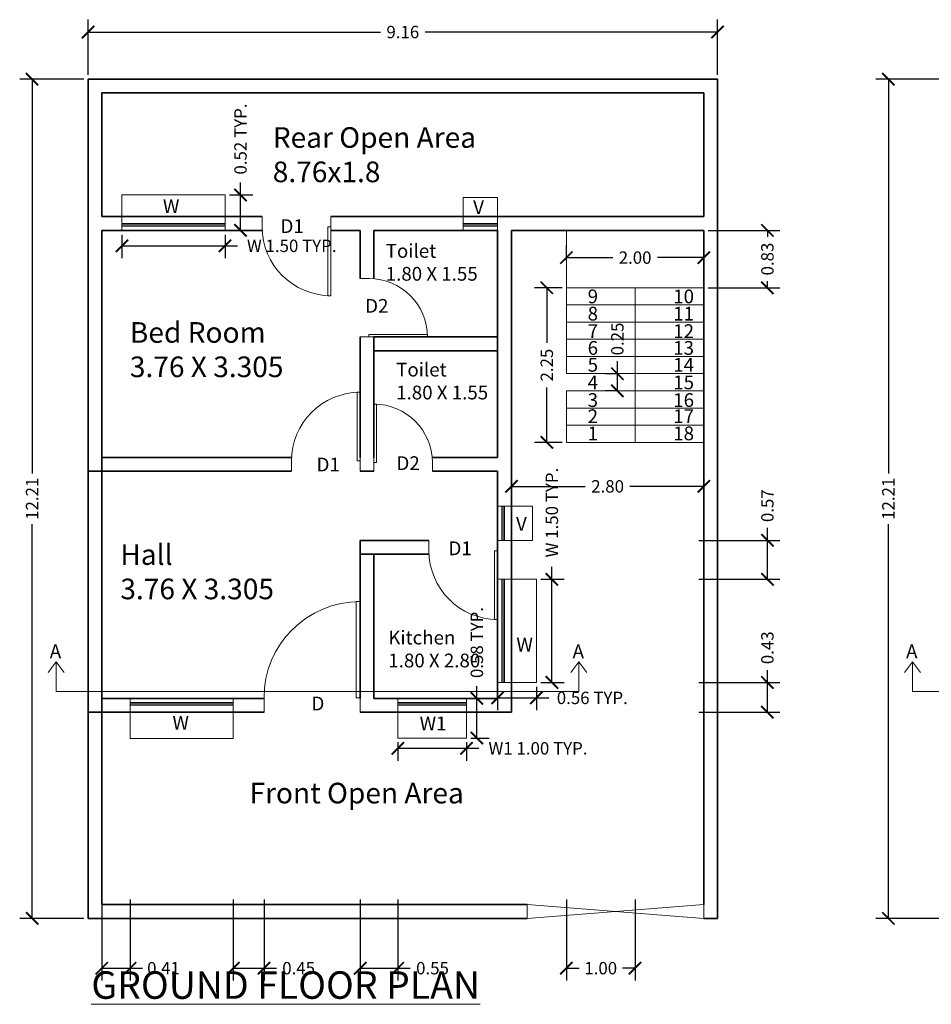
# Model space of a CAD drawing. Units: metres. Extents: x 6.8 to 74, y 0.6 to 37.
# Tile 1 of 5: x 6.8 to 20.1, y 4.1 to 18.4. Entities that reach past the tile are written whole.
import ezdxf

# ---------------------------------------------------------------- set-up
doc = ezdxf.new("R2010")
doc.units = ezdxf.units.M
doc.header["$LTSCALE"] = 0.2
doc.header["$MEASUREMENT"] = 0
for name, color, linetype, lineweight in [('A-ANNO-DIMS', 2, 'Continuous', 18), ('A-ANNO-SYMB', 3, 'Continuous', 18), ('A-ANNO-TEXT', 7, 'Continuous', 18), ('A-AREA-IDEN', 7, 'Continuous', 18), ('A-DOOR', 4, 'Continuous', 20), ('A-FLOR-STRS', 7, 'Continuous', 20), ('A-GLAZ', 4, 'Continuous', 18), ('A-WALL', 7, 'Continuous', 35)]:
    doc.layers.add(name, color=color, linetype=linetype, lineweight=lineweight)
doc.styles.get("Standard").update_dxf_attribs({"font": 'arial.ttf'})
doc.dimstyles.get("Standard").update_dxf_attribs({"dimtxt": 0.18, "dimasz": 0.18, "dimexe": 0.18, "dimexo": 0.0625, "dimgap": 0.09, "dimtad": 0, "dimzin": 0, "dimdsep": 46, "dimtxsty": 'Standard', "dimblk": 'ARCHTICK', "dimcen": 0.09, "dimadec": 0, "dimazin": 0, "dimtfac": 1, "dimtofl": 0, "dimtmove": 0, "dimatfit": 3, "dimfxl": 1, "dimfxlon": 1, "dimtolj": 1, "dimtzin": 0, "dimarcsym": 0})

# ---------------------------------------------------------------- blocks, each defined once
blk = doc.blocks.new('_ArchTick')
at = {"color": 0, "linetype": 'ByBlock', "const_width": 0.15}
blk.add_lwpolyline([(-0.5, -0.5), (0.5, 0.5)], dxfattribs=at)
blk = doc.blocks.new('*D1')
at = {"layer": 'A-ANNO-DIMS', "color": 0, "lineweight": -2, "transparency": 16777216}
for p, q in [((7.746, 17.556), (6.813, 17.556)), ((6.993, 17.556), (6.993, 11.819)), ((6.993, 5.346), (6.993, 11.083)), ((7.746, 5.346), (6.813, 5.346))]:
    blk.add_line(p, q, dxfattribs=at)
at = {"layer": 'Defpoints', "color": 0, "transparency": 16777216}
for p in [(7.808, 17.556), (6.993, 5.346), (7.808, 5.346)]:
    blk.add_point(p, dxfattribs=at)
at = {"layer": 'A-ANNO-DIMS', "color": 0, "lineweight": -2, "transparency": 16777216, "xscale": 0.18, "yscale": 0.18, "zscale": 0.18}
for p, rotation in [((6.993, 17.556), 90), ((6.993, 5.346), 270)]:
    blk.add_blockref('_ArchTick', p, dxfattribs=dict(at, rotation=rotation))
at = {"layer": 'A-ANNO-DIMS', "color": 0, "transparency": 16777216, "insert": (6.993, 11.451), "char_height": 0.18, "attachment_point": 5, "rotation": 90}
blk.add_mtext('\\A1;12.21', dxfattribs=at)
blk = doc.blocks.new('*D2')
at = {"layer": 'A-ANNO-DIMS', "color": 0, "lineweight": -2, "transparency": 16777216}
for p, q in [((7.808, 17.618), (7.808, 18.422)), ((16.968, 17.618), (16.968, 18.422)), ((7.808, 18.242), (12.064, 18.242)), ((16.968, 18.242), (12.712, 18.242))]:
    blk.add_line(p, q, dxfattribs=at)
at = {"layer": 'Defpoints', "color": 0, "transparency": 16777216}
for p in [(16.968, 18.242), (7.808, 17.556), (16.968, 17.556)]:
    blk.add_point(p, dxfattribs=at)
at = {"layer": 'A-ANNO-DIMS', "color": 0, "lineweight": -2, "transparency": 16777216, "xscale": 0.18, "yscale": 0.18, "zscale": 0.18, "rotation": 180}
blk.add_blockref('_ArchTick', (7.808, 18.242), dxfattribs=at)
at = {"layer": 'A-ANNO-DIMS', "color": 0, "lineweight": -2, "transparency": 16777216, "xscale": 0.18, "yscale": 0.18, "zscale": 0.18}
blk.add_blockref('_ArchTick', (16.968, 18.242), dxfattribs=at)
at = {"layer": 'A-ANNO-DIMS', "color": 0, "transparency": 16777216, "insert": (12.388, 18.242), "char_height": 0.18, "attachment_point": 5}
blk.add_mtext('\\A1;9.16', dxfattribs=at)
blk = doc.blocks.new('*U4')
for p, q in [((0, 0), (0, -6)), ((40, 0), (40, -6))]:
    blk.add_line(p, q)
blk.add_lwpolyline([(0, 0), (0, 40), (1.75, 40), (1.75, 0)], close=True)
blk.add_arc((0, 0), 40, 0, 90)
blk = doc.blocks.new('*D5')
at = {"layer": 'A-ANNO-DIMS', "color": 0, "lineweight": -2, "transparency": 16777216}
for p, q in [((20.206, 17.556), (19.273, 17.556)), ((19.453, 17.556), (19.453, 11.819)), ((19.453, 5.346), (19.453, 11.083)), ((20.206, 5.346), (19.273, 5.346))]:
    blk.add_line(p, q, dxfattribs=at)
at = {"layer": 'Defpoints', "color": 0, "transparency": 16777216}
for p in [(20.268, 17.556), (19.453, 5.346), (20.268, 5.346)]:
    blk.add_point(p, dxfattribs=at)
at = {"layer": 'A-ANNO-DIMS', "color": 0, "lineweight": -2, "transparency": 16777216, "xscale": 0.18, "yscale": 0.18, "zscale": 0.18}
for p, rotation in [((19.453, 17.556), 90), ((19.453, 5.346), 270)]:
    blk.add_blockref('_ArchTick', p, dxfattribs=dict(at, rotation=rotation))
at = {"layer": 'A-ANNO-DIMS', "color": 0, "transparency": 16777216, "insert": (19.453, 11.451), "char_height": 0.18, "attachment_point": 5, "rotation": 90}
blk.add_mtext('\\A1;12.21', dxfattribs=at)
blk = doc.blocks.new('*D16')
at = {"layer": 'A-ANNO-DIMS', "color": 0, "lineweight": -2, "ltscale": 0.9, "transparency": 16777216}
for p, q in [((14.768, 14.92), (14.768, 15.14)), ((16.768, 14.92), (16.768, 15.14)), ((14.768, 14.96), (15.443, 14.96)), ((16.768, 14.96), (16.093, 14.96))]:
    blk.add_line(p, q, dxfattribs=at)
at = {"layer": 'Defpoints', "color": 0, "ltscale": 0.9, "transparency": 16777216}
for p in [(16.768, 14.96), (14.768, 14.857), (16.768, 14.857)]:
    blk.add_point(p, dxfattribs=at)
at = {"layer": 'A-ANNO-DIMS', "color": 0, "lineweight": -2, "ltscale": 0.9, "transparency": 16777216, "xscale": 0.18, "yscale": 0.18, "zscale": 0.18, "rotation": 180}
blk.add_blockref('_ArchTick', (14.768, 14.96), dxfattribs=at)
at = {"layer": 'A-ANNO-DIMS', "color": 0, "lineweight": -2, "ltscale": 0.9, "transparency": 16777216, "xscale": 0.18, "yscale": 0.18, "zscale": 0.18}
blk.add_blockref('_ArchTick', (16.768, 14.96), dxfattribs=at)
at = {"layer": 'A-ANNO-DIMS', "color": 0, "ltscale": 0.9, "transparency": 16777216, "insert": (15.768, 14.96), "char_height": 0.18, "attachment_point": 5}
blk.add_mtext('\\A1;2.00', dxfattribs=at)
blk = doc.blocks.new('*D17')
at = {"layer": 'A-ANNO-DIMS', "color": 0, "lineweight": -2, "ltscale": 0.9, "transparency": 16777216}
for p, q in [((14.706, 14.521), (14.303, 14.521)), ((14.483, 14.521), (14.483, 13.722)), ((14.483, 12.271), (14.483, 13.07)), ((14.706, 12.271), (14.303, 12.271))]:
    blk.add_line(p, q, dxfattribs=at)
at = {"layer": 'Defpoints', "color": 0, "ltscale": 0.9, "transparency": 16777216}
for p in [(14.483, 14.521), (14.768, 14.521), (14.768, 12.271)]:
    blk.add_point(p, dxfattribs=at)
at = {"layer": 'A-ANNO-DIMS', "color": 0, "lineweight": -2, "ltscale": 0.9, "transparency": 16777216, "xscale": 0.18, "yscale": 0.18, "zscale": 0.18}
for p, rotation in [((14.483, 14.521), 90), ((14.483, 12.271), 270)]:
    blk.add_blockref('_ArchTick', p, dxfattribs=dict(at, rotation=rotation))
at = {"layer": 'A-ANNO-DIMS', "color": 0, "ltscale": 0.9, "transparency": 16777216, "insert": (14.483, 13.396), "char_height": 0.18, "attachment_point": 5, "rotation": 90}
blk.add_mtext('\\A1;2.25', dxfattribs=at)
blk = doc.blocks.new('*D18')
at = {"layer": 'A-ANNO-DIMS', "color": 0, "lineweight": -2, "ltscale": 0.9, "transparency": 16777216}
for p, q in [((15.51, 13.271), (15.51, 13.451)), ((15.51, 13.271), (15.33, 13.271)), ((15.51, 13.021), (15.51, 13.271)), ((15.51, 13.021), (15.33, 13.021))]:
    blk.add_line(p, q, dxfattribs=at)
at = {"layer": 'Defpoints', "color": 0, "ltscale": 0.9, "transparency": 16777216}
for p in [(15.51, 13.271), (15.51, 13.271), (15.51, 13.021)]:
    blk.add_point(p, dxfattribs=at)
at = {"layer": 'A-ANNO-DIMS', "color": 0, "lineweight": -2, "ltscale": 0.9, "transparency": 16777216, "xscale": 0.18, "yscale": 0.18, "zscale": 0.18}
for p, rotation in [((15.51, 13.271), 90), ((15.51, 13.021), 270)]:
    blk.add_blockref('_ArchTick', p, dxfattribs=dict(at, rotation=rotation))
at = {"layer": 'A-ANNO-DIMS', "color": 0, "ltscale": 0.9, "transparency": 16777216, "insert": (15.51, 13.776), "char_height": 0.18, "attachment_point": 5, "rotation": 90}
blk.add_mtext('\\A1;0.25', dxfattribs=at)
blk = doc.blocks.new('*D19')
at = {"layer": 'A-ANNO-DIMS', "color": 0, "lineweight": -2, "ltscale": 0.9, "transparency": 16777216}
for p, q in [((13.968, 11.679), (13.968, 11.452)), ((13.968, 11.632), (15.043, 11.632)), ((16.768, 11.632), (15.693, 11.632)), ((16.768, 11.679), (16.768, 11.452))]:
    blk.add_line(p, q, dxfattribs=at)
at = {"layer": 'Defpoints', "color": 0, "ltscale": 0.9, "transparency": 16777216}
for p in [(13.968, 11.741), (13.968, 11.632), (16.768, 11.741)]:
    blk.add_point(p, dxfattribs=at)
at = {"layer": 'A-ANNO-DIMS', "color": 0, "lineweight": -2, "ltscale": 0.9, "transparency": 16777216, "xscale": 0.18, "yscale": 0.18, "zscale": 0.18, "rotation": 180}
blk.add_blockref('_ArchTick', (13.968, 11.632), dxfattribs=at)
at = {"layer": 'A-ANNO-DIMS', "color": 0, "lineweight": -2, "ltscale": 0.9, "transparency": 16777216, "xscale": 0.18, "yscale": 0.18, "zscale": 0.18}
blk.add_blockref('_ArchTick', (16.768, 11.632), dxfattribs=at)
at = {"layer": 'A-ANNO-DIMS', "color": 0, "ltscale": 0.9, "transparency": 16777216, "insert": (15.368, 11.632), "char_height": 0.18, "attachment_point": 5}
blk.add_mtext('\\A1;2.80', dxfattribs=at)
blk = doc.blocks.new('WIN-W-1500-FRONT')
for p, q in [((0, 0.582), (0, 0.382)), ((1.5, 0.582), (1.5, 0.382)), ((0, 0.522), (1.5, 0.522)), ((0, 0.502), (1.5, 0.502)), ((0, 0.482), (1.5, 0.482)), ((0, 0), (0, 0.382)), ((1.5, 0.382), (1.5, 0)), ((1.5, 0), (0, 0))]:
    blk.add_line(p, q)
blk = doc.blocks.new('WIN-W1-1000-FRONT')
for p, q in [((0, 0.576), (0, 0.376)), ((1, 0.576), (1, 0.376)), ((1, 0.516), (0, 0.516)), ((1, 0.496), (0, 0.496)), ((1, 0.476), (0, 0.476)), ((0, 0), (0, 0.376)), ((1, 0.376), (1, 0)), ((1, 0), (0, 0))]:
    blk.add_line(p, q)
blk = doc.blocks.new('WIN-W-1500-SIDE')
for p, q in [((0, 1.5), (0.2, 1.5)), ((0.06, 0), (0.06, 1.5)), ((0.08, 0), (0.08, 1.5)), ((0.1, 0), (0.1, 1.5)), ((0.2, 1.5), (0.564, 1.5)), ((0.564, 1.5), (0.564, 0)), ((0, 0), (0.2, 0)), ((0.564, 0), (0.2, 0))]:
    blk.add_line(p, q)
blk = doc.blocks.new('WIN-W-1500-REAR')
for p, q in [((0, 0.2), (0, 0.517)), ((0, 0.517), (1.5, 0.517)), ((1.5, 0.517), (1.5, 0.2)), ((0, 0), (0, 0.2)), ((1.5, 0), (1.5, 0.2)), ((1.5, 0.1), (0, 0.1)), ((1.5, 0.08), (0, 0.08)), ((1.5, 0.06), (0, 0.06))]:
    blk.add_line(p, q)
blk = doc.blocks.new('VENT-500-REAR')
for p, q in [((0, 0.2), (0, 0.477)), ((0, 0.477), (0.5, 0.477)), ((0.5, 0.477), (0.5, 0.2)), ((0, 0), (0, 0.2)), ((0.5, 0), (0.5, 0.2)), ((0.5, 0.1), (0, 0.1)), ((0.5, 0.08), (0, 0.08)), ((0.5, 0.06), (0, 0.06))]:
    blk.add_line(p, q)
blk = doc.blocks.new('VENT-500-SIDE')
for p, q in [((0, 0.5), (0.2, 0.5)), ((0.06, 0.5), (0.06, 0)), ((0.08, 0.5), (0.08, 0)), ((0.1, 0.5), (0.1, 0)), ((0.2, 0.5), (0.507, 0.5)), ((0.507, 0.5), (0.507, 0)), ((0, 0), (0.2, 0)), ((0.507, 0), (0.2, 0))]:
    blk.add_line(p, q)
blk = doc.blocks.new('SECTION-HEAD-A')
for p, q in [((0, 0.429), (-0.116, 0.275)), ((0, 0), (0, 0.429)), ((0, 0.429), (0.116, 0.275))]:
    blk.add_line(p, q)
at = {"insert": (-0.093, 0.684), "char_height": 0.2, "attachment_point": 1}
blk.add_mtext_dynamic_manual_height_columns('A', width=0.50915, gutter_width=1, heights=[0], dxfattribs=at)
blk = doc.blocks.new('*D36')
at = {"layer": 'A-ANNO-DIMS', "color": 0, "lineweight": -2, "ltscale": 0.9, "transparency": 16777216}
for p, q in [((12.315, 7.908), (12.315, 7.64)), ((13.315, 7.908), (13.315, 7.64)), ((12.315, 7.82), (13.315, 7.82)), ((13.315, 7.82), (13.495, 7.82))]:
    blk.add_line(p, q, dxfattribs=at)
at = {"layer": 'Defpoints', "color": 0, "ltscale": 0.9, "transparency": 16777216}
for p in [(12.315, 7.97), (13.315, 7.97), (13.315, 7.82)]:
    blk.add_point(p, dxfattribs=at)
at = {"layer": 'A-ANNO-DIMS', "color": 0, "lineweight": -2, "ltscale": 0.9, "transparency": 16777216, "xscale": 0.18, "yscale": 0.18, "zscale": 0.18, "rotation": 180}
blk.add_blockref('_ArchTick', (12.315, 7.82), dxfattribs=at)
at = {"layer": 'A-ANNO-DIMS', "color": 0, "lineweight": -2, "ltscale": 0.9, "transparency": 16777216, "xscale": 0.18, "yscale": 0.18, "zscale": 0.18}
blk.add_blockref('_ArchTick', (13.315, 7.82), dxfattribs=at)
at = {"layer": 'A-ANNO-DIMS', "color": 0, "ltscale": 0.9, "transparency": 16777216, "insert": (14.355, 7.82), "char_height": 0.18, "attachment_point": 5}
blk.add_mtext('\\A1;W1 1.00 TYP.', dxfattribs=at)
blk = doc.blocks.new('*D37')
at = {"layer": 'A-ANNO-DIMS', "color": 0, "lineweight": -2, "ltscale": 0.9, "transparency": 16777216}
for p, q in [((13.465, 8.546), (13.465, 8.726)), ((13.378, 8.546), (13.645, 8.546)), ((13.465, 7.97), (13.465, 8.546)), ((13.378, 7.97), (13.645, 7.97))]:
    blk.add_line(p, q, dxfattribs=at)
at = {"layer": 'Defpoints', "color": 0, "ltscale": 0.9, "transparency": 16777216}
for p in [(13.315, 8.546), (13.465, 8.546), (13.315, 7.97)]:
    blk.add_point(p, dxfattribs=at)
at = {"layer": 'A-ANNO-DIMS', "color": 0, "lineweight": -2, "ltscale": 0.9, "transparency": 16777216, "xscale": 0.18, "yscale": 0.18, "zscale": 0.18}
for p, rotation in [((13.465, 8.546), 90), ((13.465, 7.97), 270)]:
    blk.add_blockref('_ArchTick', p, dxfattribs=dict(at, rotation=rotation))
at = {"layer": 'A-ANNO-DIMS', "color": 0, "ltscale": 0.9, "transparency": 16777216, "insert": (13.465, 9.359), "char_height": 0.18, "attachment_point": 5, "rotation": 90}
blk.add_mtext('\\A1;0.58 TYP.', dxfattribs=at)
blk = doc.blocks.new('*D38')
at = {"layer": 'A-ANNO-DIMS', "color": 0, "lineweight": -2, "ltscale": 0.9, "transparency": 16777216}
for p, q in [((14.557, 10.279), (14.557, 10.459)), ((14.395, 10.279), (14.737, 10.279)), ((14.557, 8.779), (14.557, 10.279)), ((14.395, 8.779), (14.737, 8.779))]:
    blk.add_line(p, q, dxfattribs=at)
at = {"layer": 'Defpoints', "color": 0, "ltscale": 0.9, "transparency": 16777216}
for p in [(14.332, 10.279), (14.557, 10.279), (14.332, 8.779)]:
    blk.add_point(p, dxfattribs=at)
at = {"layer": 'A-ANNO-DIMS', "color": 0, "lineweight": -2, "ltscale": 0.9, "transparency": 16777216, "xscale": 0.18, "yscale": 0.18, "zscale": 0.18}
for p, rotation in [((14.557, 10.279), 90), ((14.557, 8.779), 270)]:
    blk.add_blockref('_ArchTick', p, dxfattribs=dict(at, rotation=rotation))
at = {"layer": 'A-ANNO-DIMS', "color": 0, "ltscale": 0.9, "transparency": 16777216, "insert": (14.557, 11.25), "char_height": 0.18, "attachment_point": 5, "rotation": 90}
blk.add_mtext('\\A1;W 1.50 TYP.', dxfattribs=at)
blk = doc.blocks.new('*D39')
at = {"layer": 'A-ANNO-DIMS', "color": 0, "lineweight": -2, "ltscale": 0.9, "transparency": 16777216}
for p, q in [((13.768, 8.717), (13.768, 8.374)), ((14.332, 8.717), (14.332, 8.374)), ((13.768, 8.554), (14.332, 8.554)), ((14.332, 8.554), (14.512, 8.554))]:
    blk.add_line(p, q, dxfattribs=at)
at = {"layer": 'Defpoints', "color": 0, "ltscale": 0.9, "transparency": 16777216}
for p in [(13.768, 8.779), (14.332, 8.779), (14.332, 8.554)]:
    blk.add_point(p, dxfattribs=at)
at = {"layer": 'A-ANNO-DIMS', "color": 0, "lineweight": -2, "ltscale": 0.9, "transparency": 16777216, "xscale": 0.18, "yscale": 0.18, "zscale": 0.18, "rotation": 180}
blk.add_blockref('_ArchTick', (13.768, 8.554), dxfattribs=at)
at = {"layer": 'A-ANNO-DIMS', "color": 0, "lineweight": -2, "ltscale": 0.9, "transparency": 16777216, "xscale": 0.18, "yscale": 0.18, "zscale": 0.18}
blk.add_blockref('_ArchTick', (14.332, 8.554), dxfattribs=at)
at = {"layer": 'A-ANNO-DIMS', "color": 0, "ltscale": 0.9, "transparency": 16777216, "insert": (15.145, 8.554), "char_height": 0.18, "attachment_point": 5}
blk.add_mtext('\\A1;0.56 TYP.', dxfattribs=at)
blk = doc.blocks.new('*D40')
at = {"layer": 'A-ANNO-DIMS', "color": 0, "lineweight": -2, "ltscale": 0.9, "transparency": 16777216}
for p, q in [((8.301, 15.293), (8.301, 14.951)), ((9.801, 15.293), (9.801, 14.951)), ((8.301, 15.131), (9.801, 15.131)), ((9.801, 15.131), (9.981, 15.131))]:
    blk.add_line(p, q, dxfattribs=at)
at = {"layer": 'Defpoints', "color": 0, "ltscale": 0.9, "transparency": 16777216}
for p in [(8.301, 15.356), (9.801, 15.356), (9.801, 15.131)]:
    blk.add_point(p, dxfattribs=at)
at = {"layer": 'A-ANNO-DIMS', "color": 0, "lineweight": -2, "ltscale": 0.9, "transparency": 16777216, "xscale": 0.18, "yscale": 0.18, "zscale": 0.18, "rotation": 180}
blk.add_blockref('_ArchTick', (8.301, 15.131), dxfattribs=at)
at = {"layer": 'A-ANNO-DIMS', "color": 0, "lineweight": -2, "ltscale": 0.9, "transparency": 16777216, "xscale": 0.18, "yscale": 0.18, "zscale": 0.18}
blk.add_blockref('_ArchTick', (9.801, 15.131), dxfattribs=at)
at = {"layer": 'A-ANNO-DIMS', "color": 0, "ltscale": 0.9, "transparency": 16777216, "insert": (10.772, 15.131), "char_height": 0.18, "attachment_point": 5}
blk.add_mtext('\\A1;W 1.50 TYP.', dxfattribs=at)
blk = doc.blocks.new('*D41')
at = {"layer": 'A-ANNO-DIMS', "color": 0, "lineweight": -2, "ltscale": 0.9, "transparency": 16777216}
for p, q in [((10.026, 15.872), (10.026, 16.052)), ((9.864, 15.872), (10.206, 15.872)), ((10.026, 15.356), (10.026, 15.872)), ((9.864, 15.356), (10.206, 15.356))]:
    blk.add_line(p, q, dxfattribs=at)
at = {"layer": 'Defpoints', "color": 0, "ltscale": 0.9, "transparency": 16777216}
for p in [(9.801, 15.872), (10.026, 15.872), (9.801, 15.356)]:
    blk.add_point(p, dxfattribs=at)
at = {"layer": 'A-ANNO-DIMS', "color": 0, "lineweight": -2, "ltscale": 0.9, "transparency": 16777216, "xscale": 0.18, "yscale": 0.18, "zscale": 0.18}
for p, rotation in [((10.026, 15.872), 90), ((10.026, 15.356), 270)]:
    blk.add_blockref('_ArchTick', p, dxfattribs=dict(at, rotation=rotation))
at = {"layer": 'A-ANNO-DIMS', "color": 0, "ltscale": 0.9, "transparency": 16777216, "insert": (10.026, 16.685), "char_height": 0.18, "attachment_point": 5, "rotation": 90}
blk.add_mtext('\\A1;0.52 TYP.', dxfattribs=at)
blk = doc.blocks.new('*D65')
at = {"layer": 'A-ANNO-DIMS', "color": 0, "lineweight": -2, "ltscale": 0.9, "transparency": 16777216}
for p, q in [((8.008, 5.621), (8.008, 4.441)), ((8.42, 5.621), (8.42, 4.441)), ((8.008, 4.621), (8.42, 4.621)), ((8.42, 4.621), (8.6, 4.621))]:
    blk.add_line(p, q, dxfattribs=at)
at = {"layer": 'Defpoints', "color": 0, "ltscale": 0.9, "transparency": 16777216}
for p in [(8.008, 8.546), (8.42, 8.346), (8.42, 4.621)]:
    blk.add_point(p, dxfattribs=at)
at = {"layer": 'A-ANNO-DIMS', "color": 0, "lineweight": -2, "ltscale": 0.9, "transparency": 16777216, "xscale": 0.18, "yscale": 0.18, "zscale": 0.18, "rotation": 180}
blk.add_blockref('_ArchTick', (8.008, 4.621), dxfattribs=at)
at = {"layer": 'A-ANNO-DIMS', "color": 0, "lineweight": -2, "ltscale": 0.9, "transparency": 16777216, "xscale": 0.18, "yscale": 0.18, "zscale": 0.18}
blk.add_blockref('_ArchTick', (8.42, 4.621), dxfattribs=at)
at = {"layer": 'A-ANNO-DIMS', "color": 0, "ltscale": 0.9, "transparency": 16777216, "insert": (8.906, 4.621), "char_height": 0.18, "attachment_point": 5}
blk.add_mtext('\\A1;0.41', dxfattribs=at)
blk = doc.blocks.new('*D66')
at = {"layer": 'A-ANNO-DIMS', "color": 0, "lineweight": -2, "ltscale": 0.9, "transparency": 16777216}
for p, q in [((9.92, 5.621), (9.92, 4.441)), ((10.368, 5.621), (10.368, 4.441)), ((9.92, 4.621), (10.368, 4.621)), ((10.368, 4.621), (10.548, 4.621))]:
    blk.add_line(p, q, dxfattribs=at)
at = {"layer": 'Defpoints', "color": 0, "ltscale": 0.9, "transparency": 16777216}
for p in [(9.92, 8.346), (10.368, 8.346), (10.368, 4.621)]:
    blk.add_point(p, dxfattribs=at)
at = {"layer": 'A-ANNO-DIMS', "color": 0, "lineweight": -2, "ltscale": 0.9, "transparency": 16777216, "xscale": 0.18, "yscale": 0.18, "zscale": 0.18, "rotation": 180}
blk.add_blockref('_ArchTick', (9.92, 4.621), dxfattribs=at)
at = {"layer": 'A-ANNO-DIMS', "color": 0, "lineweight": -2, "ltscale": 0.9, "transparency": 16777216, "xscale": 0.18, "yscale": 0.18, "zscale": 0.18}
blk.add_blockref('_ArchTick', (10.368, 4.621), dxfattribs=at)
at = {"layer": 'A-ANNO-DIMS', "color": 0, "ltscale": 0.9, "transparency": 16777216, "insert": (10.872, 4.621), "char_height": 0.18, "attachment_point": 5}
blk.add_mtext('\\A1;0.45', dxfattribs=at)
blk = doc.blocks.new('*D67')
at = {"layer": 'A-ANNO-DIMS', "color": 0, "lineweight": -2, "ltscale": 0.9, "transparency": 16777216}
for p, q in [((11.768, 5.621), (11.768, 4.441)), ((12.315, 5.621), (12.315, 4.441)), ((11.768, 4.621), (12.315, 4.621)), ((12.315, 4.621), (12.495, 4.621))]:
    blk.add_line(p, q, dxfattribs=at)
at = {"layer": 'Defpoints', "color": 0, "ltscale": 0.9, "transparency": 16777216}
for p in [(11.768, 8.346), (12.315, 8.346), (12.315, 4.621)]:
    blk.add_point(p, dxfattribs=at)
at = {"layer": 'A-ANNO-DIMS', "color": 0, "lineweight": -2, "ltscale": 0.9, "transparency": 16777216, "xscale": 0.18, "yscale": 0.18, "zscale": 0.18, "rotation": 180}
blk.add_blockref('_ArchTick', (11.768, 4.621), dxfattribs=at)
at = {"layer": 'A-ANNO-DIMS', "color": 0, "lineweight": -2, "ltscale": 0.9, "transparency": 16777216, "xscale": 0.18, "yscale": 0.18, "zscale": 0.18}
blk.add_blockref('_ArchTick', (12.315, 4.621), dxfattribs=at)
at = {"layer": 'A-ANNO-DIMS', "color": 0, "ltscale": 0.9, "transparency": 16777216, "insert": (12.82, 4.621), "char_height": 0.18, "attachment_point": 5}
blk.add_mtext('\\A1;0.55', dxfattribs=at)
blk = doc.blocks.new('*D68')
at = {"layer": 'A-ANNO-DIMS', "color": 0, "lineweight": -2, "ltscale": 0.9, "transparency": 16777216}
for p, q in [((17.693, 8.779), (17.693, 8.959)), ((16.693, 8.779), (17.873, 8.779)), ((17.693, 8.346), (17.693, 8.779)), ((16.693, 8.346), (17.873, 8.346))]:
    blk.add_line(p, q, dxfattribs=at)
at = {"layer": 'Defpoints', "color": 0, "ltscale": 0.9, "transparency": 16777216}
for p in [(13.968, 8.779), (17.693, 8.779), (13.968, 8.346)]:
    blk.add_point(p, dxfattribs=at)
at = {"layer": 'A-ANNO-DIMS', "color": 0, "lineweight": -2, "ltscale": 0.9, "transparency": 16777216, "xscale": 0.18, "yscale": 0.18, "zscale": 0.18}
for p, rotation in [((17.693, 8.779), 90), ((17.693, 8.346), 270)]:
    blk.add_blockref('_ArchTick', p, dxfattribs=dict(at, rotation=rotation))
at = {"layer": 'A-ANNO-DIMS', "color": 0, "ltscale": 0.9, "transparency": 16777216, "insert": (17.693, 9.283), "char_height": 0.18, "attachment_point": 5, "rotation": 90}
blk.add_mtext('\\A1;0.43', dxfattribs=at)
blk = doc.blocks.new('*D69')
at = {"layer": 'A-ANNO-DIMS', "color": 0, "lineweight": -2, "ltscale": 0.9, "transparency": 16777216}
for p, q in [((17.693, 10.846), (17.693, 11.026)), ((16.693, 10.846), (17.873, 10.846)), ((17.693, 10.279), (17.693, 10.846)), ((16.693, 10.279), (17.873, 10.279))]:
    blk.add_line(p, q, dxfattribs=at)
at = {"layer": 'Defpoints', "color": 0, "ltscale": 0.9, "transparency": 16777216}
for p in [(13.968, 10.846), (17.693, 10.846), (13.968, 10.279)]:
    blk.add_point(p, dxfattribs=at)
at = {"layer": 'A-ANNO-DIMS', "color": 0, "lineweight": -2, "ltscale": 0.9, "transparency": 16777216, "xscale": 0.18, "yscale": 0.18, "zscale": 0.18}
for p, rotation in [((17.693, 10.846), 90), ((17.693, 10.279), 270)]:
    blk.add_blockref('_ArchTick', p, dxfattribs=dict(at, rotation=rotation))
at = {"layer": 'A-ANNO-DIMS', "color": 0, "ltscale": 0.9, "transparency": 16777216, "insert": (17.693, 11.35), "char_height": 0.18, "attachment_point": 5, "rotation": 90}
blk.add_mtext('\\A1;0.57', dxfattribs=at)
blk = doc.blocks.new('*D73')
at = {"layer": 'A-ANNO-DIMS', "color": 0, "lineweight": -2, "ltscale": 0.9, "transparency": 16777216}
for p, q in [((16.831, 15.356), (17.873, 15.356)), ((17.693, 15.356), (17.693, 15.262)), ((17.693, 14.521), (17.693, 14.615)), ((16.831, 14.521), (17.873, 14.521))]:
    blk.add_line(p, q, dxfattribs=at)
at = {"layer": 'Defpoints', "color": 0, "ltscale": 0.9, "transparency": 16777216}
for p in [(16.768, 15.356), (16.768, 14.521), (17.693, 14.521)]:
    blk.add_point(p, dxfattribs=at)
at = {"layer": 'A-ANNO-DIMS', "color": 0, "lineweight": -2, "ltscale": 0.9, "transparency": 16777216, "xscale": 0.18, "yscale": 0.18, "zscale": 0.18}
for p, rotation in [((17.693, 15.356), 90), ((17.693, 14.521), 270)]:
    blk.add_blockref('_ArchTick', p, dxfattribs=dict(at, rotation=rotation))
at = {"layer": 'A-ANNO-DIMS', "color": 0, "ltscale": 0.9, "transparency": 16777216, "insert": (17.693, 14.939), "char_height": 0.18, "attachment_point": 5, "rotation": 90}
blk.add_mtext('\\A1;0.83', dxfattribs=at)
blk = doc.blocks.new('*D74')
at = {"layer": 'A-ANNO-DIMS', "color": 0, "lineweight": -2, "ltscale": 0.9, "transparency": 16777216}
for p, q in [((14.768002, 5.621279), (14.768002, 4.441279)), ((15.768002, 5.621279), (15.768002, 4.441279)), ((14.768002, 4.621279), (14.953002, 4.621279)), ((15.768002, 4.621279), (15.583002, 4.621279))]:
    blk.add_line(p, q, dxfattribs=at)
at = {"layer": 'Defpoints', "color": 0, "ltscale": 0.9, "transparency": 16777216}
for p in [(14.768002, 12.27147), (15.768002, 12.27147), (15.768002, 4.621279)]:
    blk.add_point(p, dxfattribs=at)
at = {"layer": 'A-ANNO-DIMS', "color": 0, "lineweight": -2, "ltscale": 0.9, "transparency": 16777216, "xscale": 0.18, "yscale": 0.18, "zscale": 0.18, "rotation": 180}
blk.add_blockref('_ArchTick', (14.768002, 4.621279), dxfattribs=at)
at = {"layer": 'A-ANNO-DIMS', "color": 0, "lineweight": -2, "ltscale": 0.9, "transparency": 16777216, "xscale": 0.18, "yscale": 0.18, "zscale": 0.18}
blk.add_blockref('_ArchTick', (15.768002, 4.621279), dxfattribs=at)
at = {"layer": 'A-ANNO-DIMS', "color": 0, "ltscale": 0.9, "transparency": 16777216, "insert": (15.268002, 4.621279), "char_height": 0.18, "attachment_point": 5}
blk.add_mtext('\\A1;1.00', dxfattribs=at)

msp = doc.modelspace()

# ---------------------------------------------------------------- linework, layer by layer
at = {"layer": 'A-ANNO-SYMB'}
for p, q in [((14.9511, 8.6471), (7.3437, 8.6471)), ((27.4115, 8.6471), (19.8042, 8.6471))]:
    msp.add_line(p, q, dxfattribs=at)
at = {"layer": 'A-DOOR'}
for p, q in [((14.1984, 5.5458), (14.1984, 5.3458)), ((14.1984, 5.3458), (16.768, 5.5458)), ((14.1984, 5.5458), (16.768, 5.3458)), ((16.768, 5.5458), (16.768, 5.3458))]:
    msp.add_line(p, q, dxfattribs=at)
at = {"layer": 'A-FLOR-STRS'}
for p, q in [((14.768, 13.2715), (14.768, 15.3558)), ((16.768, 14.5215), (14.768, 14.5215)), ((15.768, 12.2715), (15.768, 14.5215)), ((16.768, 14.2715), (14.768, 14.2715)), ((16.768, 14.0215), (14.768, 14.0215)), ((16.768, 13.7715), (14.768, 13.7715)), ((16.768, 13.5215), (14.768, 13.5215)), ((16.768, 13.2715), (14.768, 13.2715)), ((16.768, 13.0215), (14.768, 13.0215)), ((14.768, 12.2715), (14.768, 13.0215)), ((16.768, 12.7715), (14.768, 12.7715)), ((16.768, 12.5215), (14.768, 12.5215)), ((16.768, 12.2715), (14.768, 12.2715))]:
    msp.add_line(p, q, dxfattribs=at)
at = {"layer": 'A-WALL'}
for p, q in [((7.808, 17.5558), (16.968, 17.5558)), ((7.808, 17.5558), (7.808, 5.3458)), ((16.968, 17.5558), (16.968, 5.3458)), ((8.008, 17.3558), (16.768, 17.3558)), ((8.008, 17.3558), (8.008, 15.5558)), ((16.768, 17.3558), (16.768, 15.5558)), ((8.008, 15.5558), (10.3411, 15.5558)), ((11.3411, 15.5558), (16.768, 15.5558)), ((8.008, 15.3558), (10.3423, 15.3558)), ((8.008, 15.3558), (8.008, 5.5458)), ((11.3411, 15.3558), (11.768, 15.3558)), ((11.768, 15.3558), (11.768, 14.6558)), ((11.968, 15.3558), (11.968, 14.6527)), ((11.968, 15.3558), (13.768, 15.3558)), ((13.768, 15.3558), (13.768, 12.0508)), ((13.968, 15.3558), (13.968, 8.3458)), ((13.968, 15.3558), (16.768, 15.3558)), ((16.768, 15.3558), (16.768, 5.5458)), ((11.768, 13.8058), (11.768, 12.0508)), ((11.968, 13.8058), (13.768, 13.8058)), ((11.968, 13.8058), (11.968, 12.0508)), ((11.968, 13.6058), (13.768, 13.6058)), ((8.008, 12.0508), (10.7693, 12.0508)), ((12.8149, 12.0508), (13.768, 12.0508)), ((7.808, 11.8508), (10.768, 11.8508)), ((11.768, 11.8508), (11.968, 11.8508)), ((12.818, 11.8508), (13.768, 11.8508)), ((13.768, 11.8508), (13.768, 8.5458)), ((11.768, 10.8458), (11.768, 8.5458)), ((11.768, 10.8458), (12.768, 10.8458)), ((11.768, 10.6458), (12.7693, 10.6458)), ((11.968, 10.6458), (11.968, 8.5458)), ((8.008, 8.5458), (10.368, 8.5458)), ((11.968, 8.5458), (13.768, 8.5458)), ((7.808, 8.3458), (10.368, 8.3458)), ((11.768, 8.3458), (13.968, 8.3458)), ((8.008, 5.5458), (14.1984, 5.5458)), ((7.808, 5.3458), (14.1984, 5.3458)), ((16.768, 5.3458), (16.968, 5.3458))]:
    msp.add_line(p, q, dxfattribs=at)

# ---------------------------------------------------------------- block references
at = {"layer": 'A-ANNO-SYMB'}
for p in [(7.3437, 8.6471), (14.9511, 8.6471), (19.8042, 8.6471)]:
    msp.add_blockref('SECTION-HEAD-A', p, dxfattribs=at)
at = {"layer": 'A-DOOR'}
for p, xscale, yscale, zscale, rotation in [((11.3411, 15.4058), 0.025, 0.025, 0.025, 180), ((11.8955, 13.8058), -0.02125, 0.02125, 0.02125, 270), ((13.768, 10.6958), 0.025, 0.025, 0.025, 180)]:
    msp.add_blockref('*U4', p, dxfattribs=dict(at, xscale=xscale, yscale=yscale, zscale=zscale, rotation=rotation))
for p, xscale, yscale, zscale in [((11.768, 12.0008), -0.025, 0.025, 0.025), ((11.968, 11.9783), 0.02125, 0.02125, 0.02125), ((11.768, 8.5558), -0.0350000000000001, 0.0350000000000001, 0.0350000000000001)]:
    msp.add_blockref('*U4', p, dxfattribs=dict(at, xscale=xscale, yscale=yscale, zscale=zscale))
at = {"layer": 'A-GLAZ'}
for name, p in [('WIN-W-1500-REAR', (8.3014, 15.3558)), ('VENT-500-REAR', (13.268, 15.3558)), ('VENT-500-SIDE', (13.768, 10.8458)), ('WIN-W-1500-SIDE', (13.768, 8.7794)), ('WIN-W-1500-FRONT', (8.4198, 7.9638)), ('WIN-W1-1000-FRONT', (12.3153, 7.97))]:
    msp.add_blockref(name, p, dxfattribs=at)

# ---------------------------------------------------------------- texts
at = {"layer": 'A-ANNO-TEXT', "attachment_point": 1}
for s, width, insert, char_height in [('W', 0.509148, (8.8973, 15.8073), 0.2), ('V', 0.509148, (13.4116, 15.7928), 0.2), ('D1', 0.509148, (10.6085, 15.5181), 0.2), ('9', 1.417327, (15.0776, 14.4953), 0.2), ('10', 1.417327, (16.3226, 14.4953), 0.2), ('D2', 0.509148, (11.8397, 14.3576), 0.2), ('8', 1.417327, (15.0776, 14.2442), 0.2), ('11', 1.417327, (16.3226, 14.2442), 0.2), ('7', 1.417327, (15.0776, 13.9899), 0.2), ('12', 1.417327, (16.3226, 13.9899), 0.2), ('6', 1.417327, (15.0776, 13.7457), 0.2), ('13', 1.417327, (16.3226, 13.7457), 0.2), ('5', 1.417327, (15.0776, 13.4997), 0.2), ('14', 1.417327, (16.3226, 13.4997), 0.2), ('4', 1.417327, (15.0776, 13.2441), 0.2), ('15', 1.417327, (16.3226, 13.2441), 0.2), ('3', 1.417327, (15.0776, 12.9872), 0.2), ('16', 1.417327, (16.3226, 12.9872), 0.2), ('2', 1.417327, (15.0776, 12.7522), 0.2), ('17', 1.417327, (16.3226, 12.7522), 0.2), ('1', 1.417327, (15.0776, 12.5019), 0.2), ('18', 1.417327, (16.3226, 12.5019), 0.2), ('D1', 0.509148, (11.133, 12.0492), 0.2), ('D2', 0.509148, (12.2956, 12.0693), 0.2), ('V', 0.509148, (14.035, 11.1869), 0.2), ('D1', 0.509148, (13.0529, 10.83), 0.2), ('W', 0.509148, (14.041, 9.4281), 0.2), ('D', 0.509148, (11.0592, 8.5717), 0.2), ('W', 0.509148, (9.0362, 8.2919), 0.2), ('W1', 0.509148, (12.6327, 8.2826), 0.2), ('{\\LGROUND FLOOR PLAN}', 7.004508, (7.8549, 4.5755), 0.4)]:
    msp.add_mtext_dynamic_manual_height_columns(s, width=width, gutter_width=1, heights=[0], dxfattribs=dict(at, insert=insert, char_height=char_height))
at = {"layer": 'A-AREA-IDEN', "attachment_point": 1}
for s, width, insert, char_height in [('Rear Open Area\\P8.76x1.8', 6.143632, (10.4956, 16.8575), 0.3), ('Toilet\\P1.80 X 1.55', 1.743148, (12.1391, 15.1577), 0.2), ('Bed Room\\P3.76 X 3.305', 3.423868, (8.4161, 14.0211), 0.3), ('Toilet\\P1.80 X 1.55', 1.743148, (12.2911, 13.4302), 0.2), ('Hall\\P3.76 X 3.305', 6.143632, (8.2776, 10.789), 0.3), ('Kitchen\\P1.80 X 2.80', 1.743148, (12.1765, 9.531), 0.2), ('Front Open Area', 3.328114, (10.157, 7.3187), 0.3)]:
    msp.add_mtext_dynamic_manual_height_columns(s, width=width, gutter_width=1, heights=[0], dxfattribs=dict(at, insert=insert, char_height=char_height))

# ---------------------------------------------------------------- dimensions: what is measured, and where the dimension line sits
at = {"layer": 'A-ANNO-DIMS'}
dim = msp.add_linear_dim(base=(16.968, 18.2416), p1=(7.808, 17.5558), p2=(16.968, 17.5558), dimstyle='Standard', override={"dimclrd": 0, "dimclre": 0, "dimclrt": 0}, dxfattribs=at)
dim.commit()
dim.dimension.update_dxf_attribs({"geometry": '*D2', "text_midpoint": (12.388, 18.2416)})
for base, p1, p2, picture, middle in [((6.993, 5.3458), (7.808, 17.5558), (7.808, 5.3458), '*D1', (6.993, 11.4508)), ((19.4535, 5.3458), (20.2685, 17.5558), (20.2685, 5.3458), '*D5', (19.4535, 11.4508))]:
    dim = msp.add_linear_dim(base=base, p1=p1, p2=p2, angle=90, dimstyle='Standard', override={"dimclrd": 0, "dimclre": 0, "dimclrt": 0}, dxfattribs=at)
    dim.commit()
    dim.dimension.update_dxf_attribs({"geometry": picture, "text_midpoint": middle})
at = {"layer": 'A-ANNO-DIMS', "ltscale": 0.9}
for base, p1, p2, text, picture, middle in [((10.0264, 15.8724), (9.8014, 15.3558), (9.8014, 15.8724), '<> TYP.', '*D41', (10.0264, 16.6853)), ((14.5572, 10.2794), (14.3322, 8.7794), (14.3322, 10.2794), 'W <> TYP.', '*D38', (14.5572, 11.2496)), ((13.4653, 8.5458), (13.3153, 7.97), (13.3153, 8.5458), '<> TYP.', '*D37', (13.4653, 9.3587))]:
    dim = msp.add_linear_dim(base=base, p1=p1, p2=p2, angle=90, text=text, dimstyle='Standard', override={"dimdec": 2, "dimlfac": 1, "dimrnd": 0, "dimzin": 0, "dimdsep": 46, "dimlunit": 2}, dxfattribs=at)
    dim.commit()
    dim.dimension.update_dxf_attribs({"geometry": picture, "text_midpoint": middle})
for base, p1, p2, text, picture, middle in [((9.8014, 15.1308), (8.3014, 15.3558), (9.8014, 15.3558), 'W <> TYP.', '*D40', (10.7716, 15.1308)), ((14.3322, 8.5544), (13.768, 8.7794), (14.3322, 8.7794), '<> TYP.', '*D39', (15.1452, 8.5544)), ((13.3153, 7.82), (12.3153, 7.97), (13.3153, 7.97), 'W1 <> TYP.', '*D36', (14.3554, 7.82))]:
    dim = msp.add_linear_dim(base=base, p1=p1, p2=p2, text=text, dimstyle='Standard', override={"dimdec": 2, "dimlfac": 1, "dimrnd": 0, "dimzin": 0, "dimdsep": 46, "dimlunit": 2}, dxfattribs=at)
    dim.commit()
    dim.dimension.update_dxf_attribs({"geometry": picture, "text_midpoint": middle})
for base, p1, p2, override, picture, middle in [((17.6925, 14.5215), (16.768, 15.3558), (16.768, 14.5215), {"dimdec": 2, "dimlfac": 1, "dimrnd": 0, "dimzin": 0, "dimdsep": 46, "dimlunit": 2}, '*D73', (17.6925, 14.9386)), ((14.4831, 14.5215), (14.768, 12.2715), (14.768, 14.5215), {"dimclrd": 0, "dimclre": 0, "dimclrt": 0}, '*D17', (14.4831, 13.3965)), ((15.5103, 13.2715), (15.5103, 13.0215), (15.5103, 13.2715), {"dimclrd": 0, "dimclre": 0, "dimclrt": 0}, '*D18', (15.5103, 13.7759)), ((17.6925, 10.8458), (13.968, 10.2794), (13.968, 10.8458), {"dimdec": 2, "dimlfac": 1, "dimrnd": 0, "dimzin": 0, "dimdsep": 46, "dimlunit": 2}, '*D69', (17.6925, 11.3496)), ((17.6925, 8.7794), (13.968, 8.3458), (13.968, 8.7794), {"dimdec": 2, "dimlfac": 1, "dimrnd": 0, "dimzin": 0, "dimdsep": 46, "dimlunit": 2}, '*D68', (17.6925, 9.2832))]:
    dim = msp.add_linear_dim(base=base, p1=p1, p2=p2, angle=90, dimstyle='Standard', override=override, dxfattribs=at)
    dim.commit()
    dim.dimension.update_dxf_attribs({"geometry": picture, "text_midpoint": middle})
for base, p1, p2, override, picture, middle in [((16.768, 14.9598), (14.768, 14.8572), (16.768, 14.8572), {"dimclrd": 0, "dimclre": 0, "dimclrt": 0}, '*D16', (15.768, 14.9598)), ((15.768, 4.6213), (14.768, 12.2715), (15.768, 12.2715), {"dimdec": 2, "dimlfac": 1, "dimrnd": 0, "dimzin": 0, "dimdsep": 46, "dimlunit": 2}, '*D74', (15.268, 4.6213)), ((13.968, 11.632), (16.768, 11.7414), (13.968, 11.7414), {"dimclrd": 0, "dimclre": 0, "dimclrt": 0}, '*D19', (15.368, 11.632)), ((8.4198, 4.6213), (8.008, 8.5458), (8.4198, 8.3458), {"dimdec": 2, "dimlfac": 1, "dimrnd": 0, "dimzin": 0, "dimdsep": 46, "dimlunit": 2}, '*D65', (8.9062, 4.6213)), ((10.368, 4.6213), (9.9198, 8.3458), (10.368, 8.3458), {"dimdec": 2, "dimlfac": 1, "dimrnd": 0, "dimzin": 0, "dimdsep": 46, "dimlunit": 2}, '*D66', (10.8725, 4.6213)), ((12.3153, 4.6213), (11.768, 8.3458), (12.3153, 8.3458), {"dimdec": 2, "dimlfac": 1, "dimrnd": 0, "dimzin": 0, "dimdsep": 46, "dimlunit": 2}, '*D67', (12.8197, 4.6213))]:
    dim = msp.add_linear_dim(base=base, p1=p1, p2=p2, dimstyle='Standard', override=override, dxfattribs=at)
    dim.commit()
    dim.dimension.update_dxf_attribs({"geometry": picture, "text_midpoint": middle})

doc.saveas('drawing.dxf')
